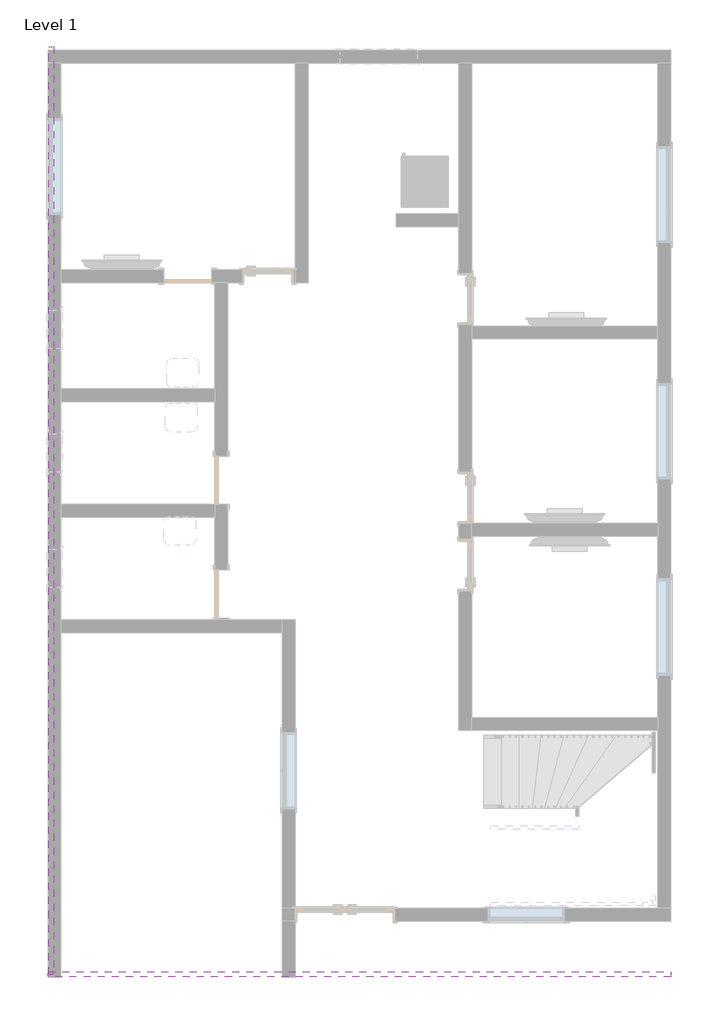
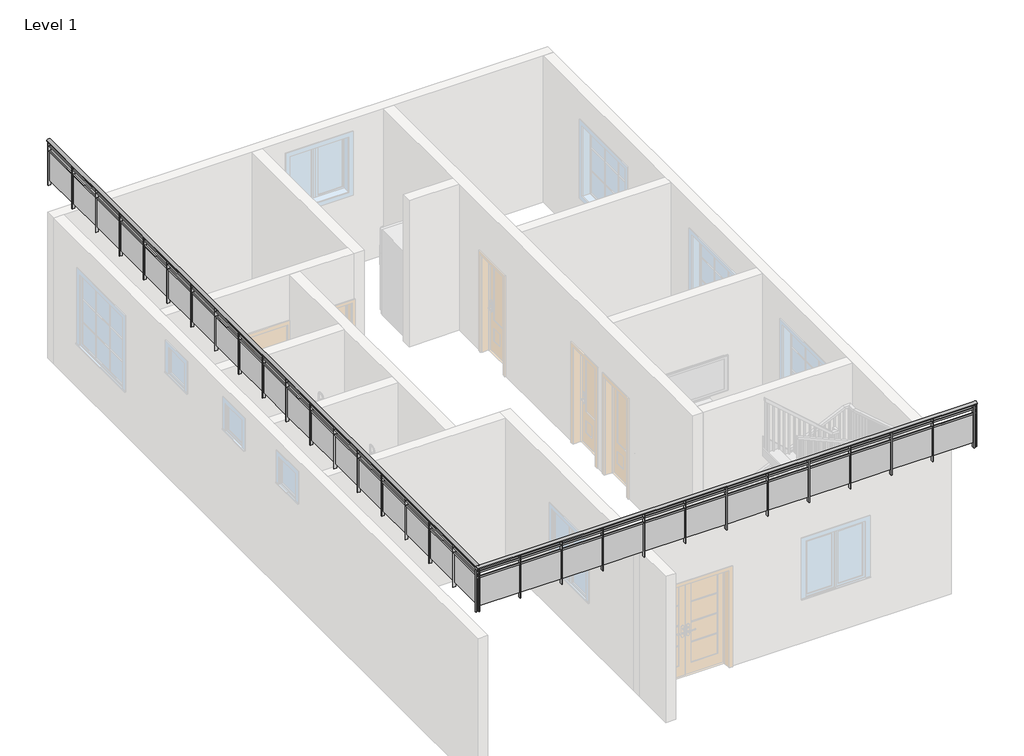
# One storey, part 2 of 4: 2 railings.
"""IFC4 building model written with IfcOpenShell, lengths in millimetres."""

from ifc_helpers import new_model, si_unit, point, frame, origin, place, context, project, spatial, polyline, ellipse_curve, trimmed, outline, extrude, element, save
from ifc_brep_helpers import plane_surface, extruded_surface, advanced_brep

model = new_model("IFC4")

# Units and contexts
model_context = context("Model", 3, world=origin())
ifc_project = project(units=[si_unit("LENGTHUNIT", "METRE", prefix="MILLI")], contexts=[model_context])

# Site, building, storey
site = spatial("IfcSite", under=ifc_project)
building = spatial("IfcBuilding", under=site)
storey = spatial("IfcBuildingStorey", under=building, Name="Level 1", Elevation=0.0)

# Railings
placement = place(None, origin())
element("IfcRailing", 1, ObjectType="Glass Panel - Bottom Fill", at=placement, inside=storey, context=model_context, shape_type="SolidModel", body=[
    advanced_brep(
    [(-12129.9047602, 13485.7174997, 4495.8), (-12206.1047602, 13485.7174997, 4495.8), (-12129.9047602, -1195.4825003, 4495.8), (-12206.1047602, -1195.4825003, 4495.8)],
    [
        (0, 1, ellipse_curve(frame((-12168.0047602, 13485.7174997, 4495.8), z_axis=(0.0, 1.0, 0.0), x_axis=(-1.0, 0.0, 0.0)), 38.1, 28.575)),
        (1, 0, ellipse_curve(frame((-12168.0047602, 13485.7174997, 4495.8), z_axis=(0.0, 1.0, 0.0), x_axis=(-1.0, 0.0, 0.0)), 38.1, 28.575)),
        (2, 3, ellipse_curve(frame((-12168.0047602, -1195.4825003, 4495.8), z_axis=(0.0, -1.0, 0.0), x_axis=(-1.0, 0.0, 0.0)), 38.1, 28.575)),
        (3, 2, ellipse_curve(frame((-12168.0047602, -1195.4825003, 4495.8), z_axis=(0.0, -1.0, 0.0), x_axis=(-1.0, 0.0, 0.0)), 38.1, 28.575)),
        (0, 2),
        (3, 1),
    ],
    [
        plane_surface(frame((-12168.0047602, 13485.7174997, 4495.8), z_axis=(0.0, 1.0, 0.0), x_axis=(0.0, 0.0, -1.0))),
        plane_surface(frame((-12168.0047602, -1195.4825003, 4495.8), z_axis=(0.0, -1.0, 0.0), x_axis=(0.0, 0.0, -1.0))),
        extruded_surface(trimmed(ellipse_curve(frame((-12168.0047602, -1195.4825003, 4495.8), z_axis=(0.0, 1.0, 0.0), x_axis=(-1.0, 0.0, 0.0)), 38.1, 28.575), [point((-12129.9047602, -1195.4825003, 4495.8))], [point((-12206.1047602, -1195.4825003, 4495.8))], True, "CARTESIAN"), (0.0, 14681.2, 0.0), 14681.2),
        extruded_surface(trimmed(ellipse_curve(frame((-12168.0047602, -1195.4825003, 4495.8), z_axis=(0.0, 1.0, 0.0), x_axis=(-1.0, 0.0, 0.0)), 38.1, 28.575), [point((-12206.1047602, -1195.4825003, 4495.8))], [point((-12129.9047602, -1195.4825003, 4495.8))], True, "CARTESIAN"), (0.0, 14681.2, 0.0), 14681.2),
    ],
    [
        (0, [[1, 2]]),
        (1, [[3, 4]]),
        (2, [[-1, 5, -4, 6]]),
        (3, [[-2, -6, -3, -5]]),
    ],
),
    extrude(outline(polyline([(-12180.7047602, 13485.7174997), (-12155.3047602, 13485.7174997), (-12155.3047602, -1195.4825003), (-12180.7047602, -1195.4825003), (-12180.7047602, 13485.7174997)])), frame((0.0, 0.0, 4381.5), z_axis=(0.0, 0.0, 1.0), x_axis=(1.0, 0.0, 0.0)), (0.0, 0.0, 1.0), 25.4),
    extrude(outline(polyline([(-12180.7047602, 13485.7174997), (-12155.3047602, 13485.7174997), (-12155.3047602, -1195.4825003), (-12180.7047602, -1195.4825003), (-12180.7047602, 13485.7174997)])), frame((0.0, 0.0, 4279.9), z_axis=(0.0, 0.0, 1.0), x_axis=(1.0, 0.0, 0.0)), (0.0, 0.0, 1.0), 25.4),
    extrude(outline(polyline([(-12193.4047602, -1163.7325003), (-12142.6047602, -1163.7325003), (-12142.6047602, -1176.4325003), (-12193.4047602, -1176.4325003), (-12193.4047602, -1163.7325003)])), frame((0.0, 0.0, 3581.4), z_axis=(0.0, 0.0, 1.0), x_axis=(1.0, 0.0, 0.0)), (0.0, 0.0, 1.0), 885.6788223),
    extrude(outline(polyline([(-12161.4696032, -357.2825003), (-12161.4696032, -1170.0825003), (-12167.8196032, -1170.0825003), (-12167.8196032, -357.2825003), (-12161.4696032, -357.2825003)])), frame((0.0, 0.0, 3683.0), z_axis=(0.0, 0.0, 1.0), x_axis=(1.0, 0.0, 0.0)), (0.0, 0.0, 1.0), 596.9),
    extrude(outline(polyline([(-12193.4047602, -350.9325003), (-12142.6047602, -350.9325003), (-12142.6047602, -363.6325003), (-12193.4047602, -363.6325003), (-12193.4047602, -350.9325003)])), frame((0.0, 0.0, 3581.4), z_axis=(0.0, 0.0, 1.0), x_axis=(1.0, 0.0, 0.0)), (0.0, 0.0, 1.0), 885.6788223),
    extrude(outline(polyline([(-12161.4696032, 455.5174997), (-12161.4696032, -357.2825003), (-12167.8196032, -357.2825003), (-12167.8196032, 455.5174997), (-12161.4696032, 455.5174997)])), frame((0.0, 0.0, 3683.0), z_axis=(0.0, 0.0, 1.0), x_axis=(1.0, 0.0, 0.0)), (0.0, 0.0, 1.0), 596.9),
    extrude(outline(polyline([(-12193.4047602, 461.8674997), (-12142.6047602, 461.8674997), (-12142.6047602, 449.1674997), (-12193.4047602, 449.1674997), (-12193.4047602, 461.8674997)])), frame((0.0, 0.0, 3581.4), z_axis=(0.0, 0.0, 1.0), x_axis=(1.0, 0.0, 0.0)), (0.0, 0.0, 1.0), 885.6788223),
    extrude(outline(polyline([(-12161.4696032, 1268.3174997), (-12161.4696032, 455.5174997), (-12167.8196032, 455.5174997), (-12167.8196032, 1268.3174997), (-12161.4696032, 1268.3174997)])), frame((0.0, 0.0, 3683.0), z_axis=(0.0, 0.0, 1.0), x_axis=(1.0, 0.0, 0.0)), (0.0, 0.0, 1.0), 596.9),
    extrude(outline(polyline([(-12193.4047602, 1274.6674997), (-12142.6047602, 1274.6674997), (-12142.6047602, 1261.9674997), (-12193.4047602, 1261.9674997), (-12193.4047602, 1274.6674997)])), frame((0.0, 0.0, 3581.4), z_axis=(0.0, 0.0, 1.0), x_axis=(1.0, 0.0, 0.0)), (0.0, 0.0, 1.0), 885.6788223),
    extrude(outline(polyline([(-12161.4696032, 2081.1174997), (-12161.4696032, 1268.3174997), (-12167.8196032, 1268.3174997), (-12167.8196032, 2081.1174997), (-12161.4696032, 2081.1174997)])), frame((0.0, 0.0, 3683.0), z_axis=(0.0, 0.0, 1.0), x_axis=(1.0, 0.0, 0.0)), (0.0, 0.0, 1.0), 596.9),
    extrude(outline(polyline([(-12193.4047602, 2087.4674997), (-12142.6047602, 2087.4674997), (-12142.6047602, 2074.7674997), (-12193.4047602, 2074.7674997), (-12193.4047602, 2087.4674997)])), frame((0.0, 0.0, 3581.4), z_axis=(0.0, 0.0, 1.0), x_axis=(1.0, 0.0, 0.0)), (0.0, 0.0, 1.0), 885.6788223),
    extrude(outline(polyline([(-12161.4696032, 2893.9174997), (-12161.4696032, 2081.1174997), (-12167.8196032, 2081.1174997), (-12167.8196032, 2893.9174997), (-12161.4696032, 2893.9174997)])), frame((0.0, 0.0, 3683.0), z_axis=(0.0, 0.0, 1.0), x_axis=(1.0, 0.0, 0.0)), (0.0, 0.0, 1.0), 596.9),
    extrude(outline(polyline([(-12193.4047602, 2900.2674997), (-12142.6047602, 2900.2674997), (-12142.6047602, 2887.5674997), (-12193.4047602, 2887.5674997), (-12193.4047602, 2900.2674997)])), frame((0.0, 0.0, 3581.4), z_axis=(0.0, 0.0, 1.0), x_axis=(1.0, 0.0, 0.0)), (0.0, 0.0, 1.0), 885.6788223),
    extrude(outline(polyline([(-12161.4696032, 3706.7174997), (-12161.4696032, 2893.9174997), (-12167.8196032, 2893.9174997), (-12167.8196032, 3706.7174997), (-12161.4696032, 3706.7174997)])), frame((0.0, 0.0, 3683.0), z_axis=(0.0, 0.0, 1.0), x_axis=(1.0, 0.0, 0.0)), (0.0, 0.0, 1.0), 596.9),
    extrude(outline(polyline([(-12193.4047602, 3713.0674997), (-12142.6047602, 3713.0674997), (-12142.6047602, 3700.3674997), (-12193.4047602, 3700.3674997), (-12193.4047602, 3713.0674997)])), frame((0.0, 0.0, 3581.4), z_axis=(0.0, 0.0, 1.0), x_axis=(1.0, 0.0, 0.0)), (0.0, 0.0, 1.0), 885.6788223),
    extrude(outline(polyline([(-12161.4696032, 4519.5174997), (-12161.4696032, 3706.7174997), (-12167.8196032, 3706.7174997), (-12167.8196032, 4519.5174997), (-12161.4696032, 4519.5174997)])), frame((0.0, 0.0, 3683.0), z_axis=(0.0, 0.0, 1.0), x_axis=(1.0, 0.0, 0.0)), (0.0, 0.0, 1.0), 596.9),
    extrude(outline(polyline([(-12193.4047602, 4525.8674997), (-12142.6047602, 4525.8674997), (-12142.6047602, 4513.1674997), (-12193.4047602, 4513.1674997), (-12193.4047602, 4525.8674997)])), frame((0.0, 0.0, 3581.4), z_axis=(0.0, 0.0, 1.0), x_axis=(1.0, 0.0, 0.0)), (0.0, 0.0, 1.0), 885.6788223),
    extrude(outline(polyline([(-12161.4696032, 5332.3174997), (-12161.4696032, 4519.5174997), (-12167.8196032, 4519.5174997), (-12167.8196032, 5332.3174997), (-12161.4696032, 5332.3174997)])), frame((0.0, 0.0, 3683.0), z_axis=(0.0, 0.0, 1.0), x_axis=(1.0, 0.0, 0.0)), (0.0, 0.0, 1.0), 596.9),
    extrude(outline(polyline([(-12193.4047602, 5338.6674997), (-12142.6047602, 5338.6674997), (-12142.6047602, 5325.9674997), (-12193.4047602, 5325.9674997), (-12193.4047602, 5338.6674997)])), frame((0.0, 0.0, 3581.4), z_axis=(0.0, 0.0, 1.0), x_axis=(1.0, 0.0, 0.0)), (0.0, 0.0, 1.0), 885.6788223),
    extrude(outline(polyline([(-12161.4696032, 6145.1174997), (-12161.4696032, 5332.3174997), (-12167.8196032, 5332.3174997), (-12167.8196032, 6145.1174997), (-12161.4696032, 6145.1174997)])), frame((0.0, 0.0, 3683.0), z_axis=(0.0, 0.0, 1.0), x_axis=(1.0, 0.0, 0.0)), (0.0, 0.0, 1.0), 596.9),
    extrude(outline(polyline([(-12193.4047602, 6151.4674997), (-12142.6047602, 6151.4674997), (-12142.6047602, 6138.7674997), (-12193.4047602, 6138.7674997), (-12193.4047602, 6151.4674997)])), frame((0.0, 0.0, 3581.4), z_axis=(0.0, 0.0, 1.0), x_axis=(1.0, 0.0, 0.0)), (0.0, 0.0, 1.0), 885.6788223),
    extrude(outline(polyline([(-12161.4696032, 6957.9174997), (-12161.4696032, 6145.1174997), (-12167.8196032, 6145.1174997), (-12167.8196032, 6957.9174997), (-12161.4696032, 6957.9174997)])), frame((0.0, 0.0, 3683.0), z_axis=(0.0, 0.0, 1.0), x_axis=(1.0, 0.0, 0.0)), (0.0, 0.0, 1.0), 596.9),
    extrude(outline(polyline([(-12193.4047602, 6964.2674997), (-12142.6047602, 6964.2674997), (-12142.6047602, 6951.5674997), (-12193.4047602, 6951.5674997), (-12193.4047602, 6964.2674997)])), frame((0.0, 0.0, 3581.4), z_axis=(0.0, 0.0, 1.0), x_axis=(1.0, 0.0, 0.0)), (0.0, 0.0, 1.0), 885.6788223),
    extrude(outline(polyline([(-12161.4696032, 7770.7174997), (-12161.4696032, 6957.9174997), (-12167.8196032, 6957.9174997), (-12167.8196032, 7770.7174997), (-12161.4696032, 7770.7174997)])), frame((0.0, 0.0, 3683.0), z_axis=(0.0, 0.0, 1.0), x_axis=(1.0, 0.0, 0.0)), (0.0, 0.0, 1.0), 596.9),
    extrude(outline(polyline([(-12193.4047602, 7777.0674997), (-12142.6047602, 7777.0674997), (-12142.6047602, 7764.3674997), (-12193.4047602, 7764.3674997), (-12193.4047602, 7777.0674997)])), frame((0.0, 0.0, 3581.4), z_axis=(0.0, 0.0, 1.0), x_axis=(1.0, 0.0, 0.0)), (0.0, 0.0, 1.0), 885.6788223),
    extrude(outline(polyline([(-12161.4696032, 8583.5174997), (-12161.4696032, 7770.7174997), (-12167.8196032, 7770.7174997), (-12167.8196032, 8583.5174997), (-12161.4696032, 8583.5174997)])), frame((0.0, 0.0, 3683.0), z_axis=(0.0, 0.0, 1.0), x_axis=(1.0, 0.0, 0.0)), (0.0, 0.0, 1.0), 596.9),
    extrude(outline(polyline([(-12193.4047602, 8589.8674997), (-12142.6047602, 8589.8674997), (-12142.6047602, 8577.1674997), (-12193.4047602, 8577.1674997), (-12193.4047602, 8589.8674997)])), frame((0.0, 0.0, 3581.4), z_axis=(0.0, 0.0, 1.0), x_axis=(1.0, 0.0, 0.0)), (0.0, 0.0, 1.0), 885.6788223),
    extrude(outline(polyline([(-12161.4696032, 9396.3174997), (-12161.4696032, 8583.5174997), (-12167.8196032, 8583.5174997), (-12167.8196032, 9396.3174997), (-12161.4696032, 9396.3174997)])), frame((0.0, 0.0, 3683.0), z_axis=(0.0, 0.0, 1.0), x_axis=(1.0, 0.0, 0.0)), (0.0, 0.0, 1.0), 596.9),
    extrude(outline(polyline([(-12193.4047602, 9402.6674997), (-12142.6047602, 9402.6674997), (-12142.6047602, 9389.9674997), (-12193.4047602, 9389.9674997), (-12193.4047602, 9402.6674997)])), frame((0.0, 0.0, 3581.4), z_axis=(0.0, 0.0, 1.0), x_axis=(1.0, 0.0, 0.0)), (0.0, 0.0, 1.0), 885.6788223),
    extrude(outline(polyline([(-12161.4696032, 10209.1174997), (-12161.4696032, 9396.3174997), (-12167.8196032, 9396.3174997), (-12167.8196032, 10209.1174997), (-12161.4696032, 10209.1174997)])), frame((0.0, 0.0, 3683.0), z_axis=(0.0, 0.0, 1.0), x_axis=(1.0, 0.0, 0.0)), (0.0, 0.0, 1.0), 596.9),
    extrude(outline(polyline([(-12193.4047602, 10215.4674997), (-12142.6047602, 10215.4674997), (-12142.6047602, 10202.7674997), (-12193.4047602, 10202.7674997), (-12193.4047602, 10215.4674997)])), frame((0.0, 0.0, 3581.4), z_axis=(0.0, 0.0, 1.0), x_axis=(1.0, 0.0, 0.0)), (0.0, 0.0, 1.0), 885.6788223),
    extrude(outline(polyline([(-12161.4696032, 11021.9174997), (-12161.4696032, 10209.1174997), (-12167.8196032, 10209.1174997), (-12167.8196032, 11021.9174997), (-12161.4696032, 11021.9174997)])), frame((0.0, 0.0, 3683.0), z_axis=(0.0, 0.0, 1.0), x_axis=(1.0, 0.0, 0.0)), (0.0, 0.0, 1.0), 596.9),
    extrude(outline(polyline([(-12193.4047602, 11028.2674997), (-12142.6047602, 11028.2674997), (-12142.6047602, 11015.5674997), (-12193.4047602, 11015.5674997), (-12193.4047602, 11028.2674997)])), frame((0.0, 0.0, 3581.4), z_axis=(0.0, 0.0, 1.0), x_axis=(1.0, 0.0, 0.0)), (0.0, 0.0, 1.0), 885.6788223),
    extrude(outline(polyline([(-12161.4696032, 11834.7174997), (-12161.4696032, 11021.9174997), (-12167.8196032, 11021.9174997), (-12167.8196032, 11834.7174997), (-12161.4696032, 11834.7174997)])), frame((0.0, 0.0, 3683.0), z_axis=(0.0, 0.0, 1.0), x_axis=(1.0, 0.0, 0.0)), (0.0, 0.0, 1.0), 596.9),
    extrude(outline(polyline([(-12193.4047602, 11841.0674997), (-12142.6047602, 11841.0674997), (-12142.6047602, 11828.3674997), (-12193.4047602, 11828.3674997), (-12193.4047602, 11841.0674997)])), frame((0.0, 0.0, 3581.4), z_axis=(0.0, 0.0, 1.0), x_axis=(1.0, 0.0, 0.0)), (0.0, 0.0, 1.0), 885.6788223),
    extrude(outline(polyline([(-12161.4696032, 12647.5174997), (-12161.4696032, 11834.7174997), (-12167.8196032, 11834.7174997), (-12167.8196032, 12647.5174997), (-12161.4696032, 12647.5174997)])), frame((0.0, 0.0, 3683.0), z_axis=(0.0, 0.0, 1.0), x_axis=(1.0, 0.0, 0.0)), (0.0, 0.0, 1.0), 596.9),
    extrude(outline(polyline([(-12193.4047602, 12653.8674997), (-12142.6047602, 12653.8674997), (-12142.6047602, 12641.1674997), (-12193.4047602, 12641.1674997), (-12193.4047602, 12653.8674997)])), frame((0.0, 0.0, 3581.4), z_axis=(0.0, 0.0, 1.0), x_axis=(1.0, 0.0, 0.0)), (0.0, 0.0, 1.0), 885.6788223),
    extrude(outline(polyline([(-12161.4696032, 13460.3174997), (-12161.4696032, 12647.5174997), (-12167.8196032, 12647.5174997), (-12167.8196032, 13460.3174997), (-12161.4696032, 13460.3174997)])), frame((0.0, 0.0, 3683.0), z_axis=(0.0, 0.0, 1.0), x_axis=(1.0, 0.0, 0.0)), (0.0, 0.0, 1.0), 596.9),
    extrude(outline(polyline([(-12193.4047602, 13466.6674997), (-12142.6047602, 13466.6674997), (-12142.6047602, 13453.9674997), (-12193.4047602, 13453.9674997), (-12193.4047602, 13466.6674997)])), frame((0.0, 0.0, 3581.4), z_axis=(0.0, 0.0, 1.0), x_axis=(1.0, 0.0, 0.0)), (0.0, 0.0, 1.0), 885.6788223),
    extrude(outline(polyline([(-12177.5297602, -1182.7825003), (-12158.4797602, -1182.7825003), (-12158.4797602, -1201.8325003), (-12177.5297602, -1201.8325003), (-12177.5297602, -1182.7825003)])), frame((0.0, 0.0, 3581.4), z_axis=(0.0, 0.0, 1.0), x_axis=(1.0, 0.0, 0.0)), (0.0, 0.0, 1.0), 885.6788223),
    extrude(outline(polyline([(-12177.5297602, 13492.0674997), (-12158.4797602, 13492.0674997), (-12158.4797602, 13473.0174997), (-12177.5297602, 13473.0174997), (-12177.5297602, 13492.0674997)])), frame((0.0, 0.0, 3581.4), z_axis=(0.0, 0.0, 1.0), x_axis=(1.0, 0.0, 0.0)), (0.0, 0.0, 1.0), 885.6788223),
])
element("IfcRailing", 2, ObjectType="Glass Panel - Bottom Fill", at=placement, inside=storey, context=model_context, shape_type="SolidModel", body=[
    advanced_brep(
    [(-12218.8047602, -1157.3825003, 4495.8), (-12218.8047602, -1233.5825003, 4495.8), (-2363.6047602, -1157.3825003, 4495.8), (-2363.6047602, -1233.5825003, 4495.8)],
    [
        (0, 1, ellipse_curve(frame((-12218.8047602, -1195.4825003, 4495.8), z_axis=(-1.0, 0.0, 0.0), x_axis=(0.0, -1.0, 0.0)), 38.1, 28.575)),
        (1, 0, ellipse_curve(frame((-12218.8047602, -1195.4825003, 4495.8), z_axis=(-1.0, 0.0, 0.0), x_axis=(0.0, -1.0, 0.0)), 38.1, 28.575)),
        (2, 3, ellipse_curve(frame((-2363.6047602, -1195.4825003, 4495.8), z_axis=(1.0, 0.0, 0.0), x_axis=(0.0, -1.0, 0.0)), 38.1, 28.575)),
        (3, 2, ellipse_curve(frame((-2363.6047602, -1195.4825003, 4495.8), z_axis=(1.0, 0.0, 0.0), x_axis=(0.0, -1.0, 0.0)), 38.1, 28.575)),
        (0, 2),
        (3, 1),
    ],
    [
        plane_surface(frame((-12218.8047602, -1195.4825003, 4495.8), z_axis=(-1.0, 0.0, 0.0), x_axis=(0.0, 1.0, 0.0))),
        plane_surface(frame((-2363.6047602, -1195.4825003, 4495.8), z_axis=(1.0, 0.0, 0.0), x_axis=(0.0, 1.0, 0.0))),
        extruded_surface(trimmed(ellipse_curve(frame((-2363.6047602, -1195.4825003, 4495.8), z_axis=(-1.0, 0.0, 0.0), x_axis=(0.0, -1.0, 0.0)), 38.1, 28.575), [point((-2363.6047602, -1157.3825003, 4495.8))], [point((-2363.6047602, -1233.5825003, 4495.8))], True, "CARTESIAN"), (-9855.2, 0.0, 0.0), 9855.2),
        extruded_surface(trimmed(ellipse_curve(frame((-2363.6047602, -1195.4825003, 4495.8), z_axis=(-1.0, 0.0, 0.0), x_axis=(0.0, -1.0, 0.0)), 38.1, 28.575), [point((-2363.6047602, -1233.5825003, 4495.8))], [point((-2363.6047602, -1157.3825003, 4495.8))], True, "CARTESIAN"), (-9855.2, 0.0, 0.0), 9855.2),
    ],
    [
        (0, [[1, 2]]),
        (1, [[3, 4]]),
        (2, [[-1, 5, -4, 6]]),
        (3, [[-2, -6, -3, -5]]),
    ],
),
    extrude(outline(polyline([(-12218.8047602, -1208.1825003), (-12218.8047602, -1182.7825003), (-2363.6047602, -1182.7825003), (-2363.6047602, -1208.1825003), (-12218.8047602, -1208.1825003)])), frame((0.0, 0.0, 4381.5), z_axis=(0.0, 0.0, 1.0), x_axis=(1.0, 0.0, 0.0)), (0.0, 0.0, 1.0), 25.4),
    extrude(outline(polyline([(-12218.8047602, -1208.1825003), (-12218.8047602, -1182.7825003), (-2363.6047602, -1182.7825003), (-2363.6047602, -1208.1825003), (-12218.8047602, -1208.1825003)])), frame((0.0, 0.0, 4279.9), z_axis=(0.0, 0.0, 1.0), x_axis=(1.0, 0.0, 0.0)), (0.0, 0.0, 1.0), 25.4),
    extrude(outline(polyline([(-2420.7547602, -1220.8825003), (-2420.7547602, -1170.0825003), (-2408.0547602, -1170.0825003), (-2408.0547602, -1220.8825003), (-2420.7547602, -1220.8825003)])), frame((0.0, 0.0, 3581.4), z_axis=(0.0, 0.0, 1.0), x_axis=(1.0, 0.0, 0.0)), (0.0, 0.0, 1.0), 885.6788223),
    extrude(outline(polyline([(-3227.2047602, -1188.9473433), (-2414.4047602, -1188.9473433), (-2414.4047602, -1195.2973433), (-3227.2047602, -1195.2973433), (-3227.2047602, -1188.9473433)])), frame((0.0, 0.0, 3683.0), z_axis=(0.0, 0.0, 1.0), x_axis=(1.0, 0.0, 0.0)), (0.0, 0.0, 1.0), 596.9),
    extrude(outline(polyline([(-3233.5547602, -1220.8825003), (-3233.5547602, -1170.0825003), (-3220.8547602, -1170.0825003), (-3220.8547602, -1220.8825003), (-3233.5547602, -1220.8825003)])), frame((0.0, 0.0, 3581.4), z_axis=(0.0, 0.0, 1.0), x_axis=(1.0, 0.0, 0.0)), (0.0, 0.0, 1.0), 885.6788223),
    extrude(outline(polyline([(-4040.0047602, -1188.9473433), (-3227.2047602, -1188.9473433), (-3227.2047602, -1195.2973433), (-4040.0047602, -1195.2973433), (-4040.0047602, -1188.9473433)])), frame((0.0, 0.0, 3683.0), z_axis=(0.0, 0.0, 1.0), x_axis=(1.0, 0.0, 0.0)), (0.0, 0.0, 1.0), 596.9),
    extrude(outline(polyline([(-4046.3547602, -1220.8825003), (-4046.3547602, -1170.0825003), (-4033.6547602, -1170.0825003), (-4033.6547602, -1220.8825003), (-4046.3547602, -1220.8825003)])), frame((0.0, 0.0, 3581.4), z_axis=(0.0, 0.0, 1.0), x_axis=(1.0, 0.0, 0.0)), (0.0, 0.0, 1.0), 885.6788223),
    extrude(outline(polyline([(-4852.8047602, -1188.9473433), (-4040.0047602, -1188.9473433), (-4040.0047602, -1195.2973433), (-4852.8047602, -1195.2973433), (-4852.8047602, -1188.9473433)])), frame((0.0, 0.0, 3683.0), z_axis=(0.0, 0.0, 1.0), x_axis=(1.0, 0.0, 0.0)), (0.0, 0.0, 1.0), 596.9),
    extrude(outline(polyline([(-4859.1547602, -1220.8825003), (-4859.1547602, -1170.0825003), (-4846.4547602, -1170.0825003), (-4846.4547602, -1220.8825003), (-4859.1547602, -1220.8825003)])), frame((0.0, 0.0, 3581.4), z_axis=(0.0, 0.0, 1.0), x_axis=(1.0, 0.0, 0.0)), (0.0, 0.0, 1.0), 885.6788223),
    extrude(outline(polyline([(-5665.6047602, -1188.9473433), (-4852.8047602, -1188.9473433), (-4852.8047602, -1195.2973433), (-5665.6047602, -1195.2973433), (-5665.6047602, -1188.9473433)])), frame((0.0, 0.0, 3683.0), z_axis=(0.0, 0.0, 1.0), x_axis=(1.0, 0.0, 0.0)), (0.0, 0.0, 1.0), 596.9),
    extrude(outline(polyline([(-5671.9547602, -1220.8825003), (-5671.9547602, -1170.0825003), (-5659.2547602, -1170.0825003), (-5659.2547602, -1220.8825003), (-5671.9547602, -1220.8825003)])), frame((0.0, 0.0, 3581.4), z_axis=(0.0, 0.0, 1.0), x_axis=(1.0, 0.0, 0.0)), (0.0, 0.0, 1.0), 885.6788223),
    extrude(outline(polyline([(-6478.4047602, -1188.9473433), (-5665.6047602, -1188.9473433), (-5665.6047602, -1195.2973433), (-6478.4047602, -1195.2973433), (-6478.4047602, -1188.9473433)])), frame((0.0, 0.0, 3683.0), z_axis=(0.0, 0.0, 1.0), x_axis=(1.0, 0.0, 0.0)), (0.0, 0.0, 1.0), 596.9),
    extrude(outline(polyline([(-6484.7547602, -1220.8825003), (-6484.7547602, -1170.0825003), (-6472.0547602, -1170.0825003), (-6472.0547602, -1220.8825003), (-6484.7547602, -1220.8825003)])), frame((0.0, 0.0, 3581.4), z_axis=(0.0, 0.0, 1.0), x_axis=(1.0, 0.0, 0.0)), (0.0, 0.0, 1.0), 885.6788223),
    extrude(outline(polyline([(-7291.2047602, -1188.9473433), (-6478.4047602, -1188.9473433), (-6478.4047602, -1195.2973433), (-7291.2047602, -1195.2973433), (-7291.2047602, -1188.9473433)])), frame((0.0, 0.0, 3683.0), z_axis=(0.0, 0.0, 1.0), x_axis=(1.0, 0.0, 0.0)), (0.0, 0.0, 1.0), 596.9),
    extrude(outline(polyline([(-7297.5547602, -1220.8825003), (-7297.5547602, -1170.0825003), (-7284.8547602, -1170.0825003), (-7284.8547602, -1220.8825003), (-7297.5547602, -1220.8825003)])), frame((0.0, 0.0, 3581.4), z_axis=(0.0, 0.0, 1.0), x_axis=(1.0, 0.0, 0.0)), (0.0, 0.0, 1.0), 885.6788223),
    extrude(outline(polyline([(-8104.0047602, -1188.9473433), (-7291.2047602, -1188.9473433), (-7291.2047602, -1195.2973433), (-8104.0047602, -1195.2973433), (-8104.0047602, -1188.9473433)])), frame((0.0, 0.0, 3683.0), z_axis=(0.0, 0.0, 1.0), x_axis=(1.0, 0.0, 0.0)), (0.0, 0.0, 1.0), 596.9),
    extrude(outline(polyline([(-8110.3547602, -1220.8825003), (-8110.3547602, -1170.0825003), (-8097.6547602, -1170.0825003), (-8097.6547602, -1220.8825003), (-8110.3547602, -1220.8825003)])), frame((0.0, 0.0, 3581.4), z_axis=(0.0, 0.0, 1.0), x_axis=(1.0, 0.0, 0.0)), (0.0, 0.0, 1.0), 885.6788223),
    extrude(outline(polyline([(-8916.8047602, -1188.9473433), (-8104.0047602, -1188.9473433), (-8104.0047602, -1195.2973433), (-8916.8047602, -1195.2973433), (-8916.8047602, -1188.9473433)])), frame((0.0, 0.0, 3683.0), z_axis=(0.0, 0.0, 1.0), x_axis=(1.0, 0.0, 0.0)), (0.0, 0.0, 1.0), 596.9),
    extrude(outline(polyline([(-8923.1547602, -1220.8825003), (-8923.1547602, -1170.0825003), (-8910.4547602, -1170.0825003), (-8910.4547602, -1220.8825003), (-8923.1547602, -1220.8825003)])), frame((0.0, 0.0, 3581.4), z_axis=(0.0, 0.0, 1.0), x_axis=(1.0, 0.0, 0.0)), (0.0, 0.0, 1.0), 885.6788223),
    extrude(outline(polyline([(-9729.6047602, -1188.9473433), (-8916.8047602, -1188.9473433), (-8916.8047602, -1195.2973433), (-9729.6047602, -1195.2973433), (-9729.6047602, -1188.9473433)])), frame((0.0, 0.0, 3683.0), z_axis=(0.0, 0.0, 1.0), x_axis=(1.0, 0.0, 0.0)), (0.0, 0.0, 1.0), 596.9),
    extrude(outline(polyline([(-9735.9547602, -1220.8825003), (-9735.9547602, -1170.0825003), (-9723.2547602, -1170.0825003), (-9723.2547602, -1220.8825003), (-9735.9547602, -1220.8825003)])), frame((0.0, 0.0, 3581.4), z_axis=(0.0, 0.0, 1.0), x_axis=(1.0, 0.0, 0.0)), (0.0, 0.0, 1.0), 885.6788223),
    extrude(outline(polyline([(-10542.4047602, -1188.9473433), (-9729.6047602, -1188.9473433), (-9729.6047602, -1195.2973433), (-10542.4047602, -1195.2973433), (-10542.4047602, -1188.9473433)])), frame((0.0, 0.0, 3683.0), z_axis=(0.0, 0.0, 1.0), x_axis=(1.0, 0.0, 0.0)), (0.0, 0.0, 1.0), 596.9),
    extrude(outline(polyline([(-10548.7547602, -1220.8825003), (-10548.7547602, -1170.0825003), (-10536.0547602, -1170.0825003), (-10536.0547602, -1220.8825003), (-10548.7547602, -1220.8825003)])), frame((0.0, 0.0, 3581.4), z_axis=(0.0, 0.0, 1.0), x_axis=(1.0, 0.0, 0.0)), (0.0, 0.0, 1.0), 885.6788223),
    extrude(outline(polyline([(-11355.2047602, -1188.9473433), (-10542.4047602, -1188.9473433), (-10542.4047602, -1195.2973433), (-11355.2047602, -1195.2973433), (-11355.2047602, -1188.9473433)])), frame((0.0, 0.0, 3683.0), z_axis=(0.0, 0.0, 1.0), x_axis=(1.0, 0.0, 0.0)), (0.0, 0.0, 1.0), 596.9),
    extrude(outline(polyline([(-11361.5547602, -1220.8825003), (-11361.5547602, -1170.0825003), (-11348.8547602, -1170.0825003), (-11348.8547602, -1220.8825003), (-11361.5547602, -1220.8825003)])), frame((0.0, 0.0, 3581.4), z_axis=(0.0, 0.0, 1.0), x_axis=(1.0, 0.0, 0.0)), (0.0, 0.0, 1.0), 885.6788223),
    extrude(outline(polyline([(-12168.0047602, -1188.9473433), (-11355.2047602, -1188.9473433), (-11355.2047602, -1195.2973433), (-12168.0047602, -1195.2973433), (-12168.0047602, -1188.9473433)])), frame((0.0, 0.0, 3683.0), z_axis=(0.0, 0.0, 1.0), x_axis=(1.0, 0.0, 0.0)), (0.0, 0.0, 1.0), 596.9),
    extrude(outline(polyline([(-12174.3547602, -1220.8825003), (-12174.3547602, -1170.0825003), (-12161.6547602, -1170.0825003), (-12161.6547602, -1220.8825003), (-12174.3547602, -1220.8825003)])), frame((0.0, 0.0, 3581.4), z_axis=(0.0, 0.0, 1.0), x_axis=(1.0, 0.0, 0.0)), (0.0, 0.0, 1.0), 885.6788223),
    extrude(outline(polyline([(-2376.3047602, -1205.0075003), (-2376.3047602, -1185.9575003), (-2357.2547602, -1185.9575003), (-2357.2547602, -1205.0075003), (-2376.3047602, -1205.0075003)])), frame((0.0, 0.0, 3581.4), z_axis=(0.0, 0.0, 1.0), x_axis=(1.0, 0.0, 0.0)), (0.0, 0.0, 1.0), 885.6788223),
    extrude(outline(polyline([(-12225.1547602, -1205.0075003), (-12225.1547602, -1185.9575003), (-12206.1047602, -1185.9575003), (-12206.1047602, -1205.0075003), (-12225.1547602, -1205.0075003)])), frame((0.0, 0.0, 3581.4), z_axis=(0.0, 0.0, 1.0), x_axis=(1.0, 0.0, 0.0)), (0.0, 0.0, 1.0), 885.6788223),
])

save(model, "model.ifc")

# Revit data of these elements
# Type "Glass Panel - Bottom Fill"
#   Assembly Code = "C2010400"
#   built-in parameter 1008612 = 0.0416667 (stored number, unit not read)
#   built-in parameter 1008611 = 0.0416667 (stored number, unit not read)
#   built-in parameter 1008609 = 0.333333 (stored number, unit not read)
#   built-in parameter 1008604 = 0.166667 (stored number, unit not read)
#   built-in parameter 1008603 = 0.166667 (stored number, unit not read)
#   Railing Height = 3' - 0"
#   built-in parameter 1008630 = 2
#   built-in parameter 1008610 = 2
#   built-in parameter 1008618 = Baluster - Square : 3/4"
# Elements 1, 2 (IfcRailing, "Glass Panel - Bottom Fill")
#   built-in parameter 1008621 = 11.75 (stored number, unit not read)
#   Phase Created = New Construction
#   Materials on its faces: "Glass"
# Materials
#   "Glass": class "Glass", colour RGB 0 128 192, transparency 0.75, Description = "Soda Lime Glass", Cost = 0
